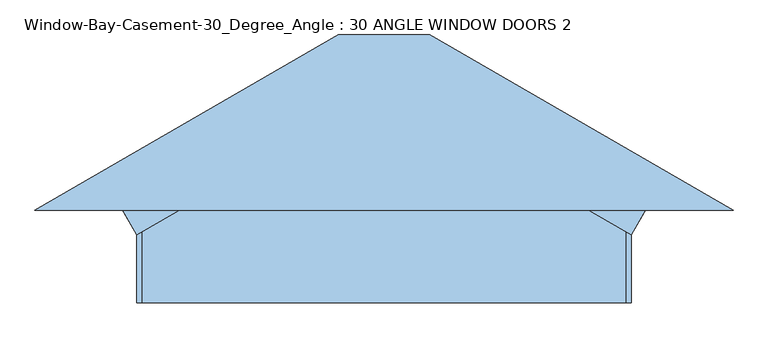
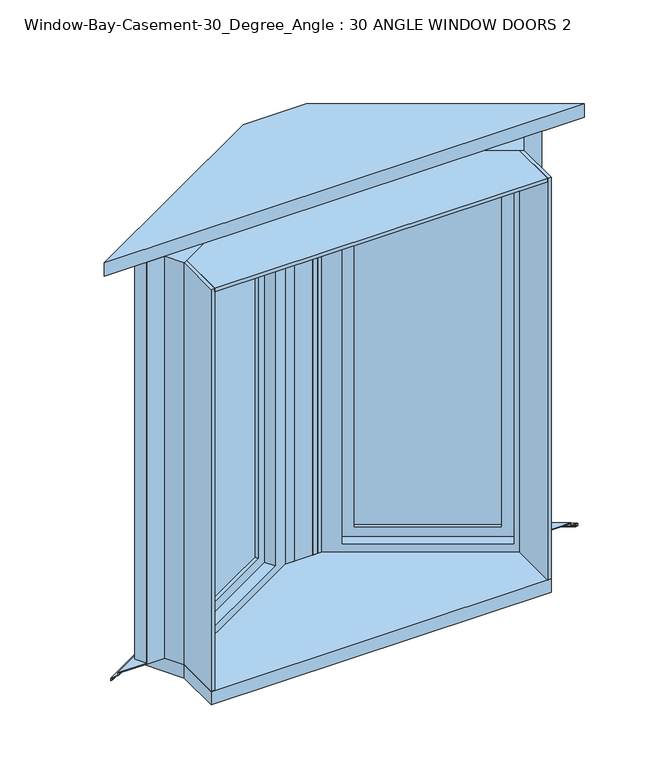
"""IFC4 building model written with IfcOpenShell, lengths in millimetres: window geometry, Window-Bay-Casement-30_Degree_Angle : 30 ANGLE WINDOW DOORS 2."""

from ifc_helpers import new_model, si_unit, frame, origin, place, context, project, spatial, polyline, outline, extrude, faceted_brep, source, transform, mapped, element, save


def window_bay_casement_30_degree_angle_30_angle_window_doors_2_b97d1700(model_context):
    return source(origin(), model_context, "Body", "SolidModel", [
        extrude(outline(polyline([(584.0331255, 149.225), (580.8581255, 143.7257387), (184.9113109, 372.3257387), (188.0863109, 377.825), (584.0331255, 149.225)])), frame((0.0, 0.0, 730.25), z_axis=(0.0, 0.0, 1.0), x_axis=(1.0, 0.0, 0.0)), (0.0, 0.0, 1.0), 1384.3),
        extrude(outline(polyline([(577.6831255, 138.2264774), (574.5081255, 132.7272161), (178.5613109, 361.3272161), (181.7363109, 366.8264774), (577.6831255, 138.2264774)])), frame((0.0, 0.0, 730.25), z_axis=(0.0, 0.0, 1.0), x_axis=(1.0, 0.0, 0.0)), (0.0, 0.0, 1.0), 1384.3),
        extrude(outline(polyline([(1441.45, 57.1500001), (1441.45, -514.35), (-57.15, -514.35), (-57.15, 57.1500001), (1441.45, 57.1500001)]), holes=[polyline([(1384.3, -457.2), (1384.3, 0.0), (0.0, 0.0), (0.0, -457.2), (1384.3, -457.2)])]), frame((568.1581255, 121.7286934, 730.25), z_axis=(0.49999999999999967, 0.8660254037844389, 0.0), x_axis=(0.0, 0.0, 1.0)), (0.0, 0.0, 1.0), 44.45),
        faceted_brep([(64.8840949, 368.3, 2184.4), (609.6, 53.8081255, 2184.4), (644.525, 114.3, 2184.4), (708.025, 114.3, 2184.4), (92.1077328, 469.9, 2184.4), (617.6514774, 93.1536934, 2171.7), (122.7179591, 378.9036934, 2171.7), (154.4679591, 433.8963066, 2171.7), (649.4014774, 148.1463066, 2171.7), (582.1036934, 69.6831255, 2152.65), (120.1657431, 336.3831255, 2152.65), (139.2157431, 369.3786934, 2152.65), (601.1536934, 102.6786934, 2152.65), (122.7179591, 378.9036934, 673.1), (154.4679591, 433.8963066, 673.1), (120.1657431, 336.3831255, 692.15), (139.2157431, 369.3786934, 692.15), (92.1077328, 469.9, 660.4), (708.025, 114.3, 660.4), (644.525, 114.3, 660.4), (609.6, 53.8081255, 660.4), (64.8840949, 368.3, 660.4), (617.6514774, 93.1536934, 673.1), (649.4014774, 148.1463066, 673.1), (582.1036934, 69.6831255, 692.15), (601.1536934, 102.6786934, 692.15)], [[[0, 1, 2, 3, 4]], [[5, 6, 7, 8]], [[9, 10, 11, 12]], [[6, 13, 14, 7]], [[10, 15, 16, 11]], [[17, 18, 19, 20, 21]], [[13, 22, 23, 14]], [[15, 24, 25, 16]], [[20, 19, 2, 1]], [[3, 18, 17, 4], [7, 14, 23, 8]], [[8, 23, 22, 5]], [[5, 22, 13, 6], [11, 16, 25, 12]], [[12, 25, 24, 9]], [[1, 0, 21, 20], [9, 24, 15, 10]], [[4, 17, 21, 0]], [[2, 19, 18, 3]]]),
        extrude(outline(polyline([(-584.0331255, 149.225), (-188.0863109, 377.825), (-184.9113109, 372.3257387), (-580.8581255, 143.7257387), (-584.0331255, 149.225)])), frame((0.0, 0.0, 730.25), z_axis=(0.0, 0.0, 1.0), x_axis=(1.0, 0.0, 0.0)), (0.0, 0.0, 1.0), 1384.3),
        extrude(outline(polyline([(-577.6831255, 138.2264774), (-181.7363109, 366.8264774), (-178.5613109, 361.3272161), (-574.5081255, 132.7272161), (-577.6831255, 138.2264774)])), frame((0.0, 0.0, 730.25), z_axis=(0.0, 0.0, 1.0), x_axis=(1.0, 0.0, 0.0)), (0.0, 0.0, 1.0), 1384.3),
        extrude(outline(polyline([(1441.45, -57.1500001), (-57.15, -57.1500001), (-57.15, 514.35), (1441.45, 514.35), (1441.45, -57.1500001)]), holes=[polyline([(1384.3, 457.2), (0.0, 457.2), (0.0, 0.0), (1384.3, 0.0), (1384.3, 457.2)])]), frame((-568.1581255, 121.7286934, 730.25), z_axis=(-0.49999999999999967, 0.8660254037844389, 0.0), x_axis=(0.0, 0.0, 1.0)), (0.0, 0.0, 1.0), 44.45),
        faceted_brep([(-64.8840949, 368.3, 2184.4), (-92.1077328, 469.9, 2184.4), (-708.025, 114.3, 2184.4), (-644.525, 114.3, 2184.4), (-609.6, 53.8081255, 2184.4), (-617.6514774, 93.1536934, 2171.7), (-649.4014774, 148.1463066, 2171.7), (-154.4679591, 433.8963066, 2171.7), (-122.7179591, 378.9036934, 2171.7), (-582.1036934, 69.6831255, 2152.65), (-601.1536934, 102.6786934, 2152.65), (-139.2157431, 369.3786934, 2152.65), (-120.1657431, 336.3831255, 2152.65), (-154.4679591, 433.8963066, 673.1), (-122.7179591, 378.9036934, 673.1), (-139.2157431, 369.3786934, 692.15), (-120.1657431, 336.3831255, 692.15), (-92.1077328, 469.9, 660.4), (-64.8840949, 368.3, 660.4), (-609.6, 53.8081255, 660.4), (-644.525, 114.3, 660.4), (-708.025, 114.3, 660.4), (-649.4014774, 148.1463066, 673.1), (-617.6514774, 93.1536934, 673.1), (-601.1536934, 102.6786934, 692.15), (-582.1036934, 69.6831255, 692.15)], [[[0, 1, 2, 3, 4]], [[5, 6, 7, 8]], [[9, 10, 11, 12]], [[8, 7, 13, 14]], [[12, 11, 15, 16]], [[17, 18, 19, 20, 21]], [[14, 13, 22, 23]], [[16, 15, 24, 25]], [[19, 4, 3, 20]], [[2, 1, 17, 21], [7, 6, 22, 13]], [[6, 5, 23, 22]], [[5, 8, 14, 23], [11, 10, 24, 15]], [[10, 9, 25, 24]], [[4, 19, 18, 0], [9, 12, 16, 25]], [[1, 0, 18, 17]], [[3, 2, 21, 20]]]),
        faceted_brep([(-105.7449774, 520.7, 660.4), (-105.7449774, 520.7, 653.0697935), (105.7449774, 520.7, 653.0697935), (105.7449774, 520.7, 660.4), (-92.1331585, 469.9, 663.1486341), (-92.1331585, 469.9, 660.4), (92.1331585, 469.9, 660.4), (92.1331585, 469.9, 663.1486341), (-106.1193025, 522.097, 654.4483503), (-106.1193025, 522.097, 663.1486341), (106.1193025, 522.097, 663.1486341), (106.1193025, 522.097, 654.4483503), (109.5222572, 534.797, 652.2089977), (-109.5222572, 534.797, 652.2089977), (109.5222572, 534.797, 643.2668038), (-109.5222572, 534.797, 643.2668038), (-108.4605353, 530.8346, 644.7270038), (-108.4605353, 530.8346, 643.2668038), (108.4605353, 530.8346, 643.2668038), (108.4605353, 530.8346, 644.7270038), (-109.0934849, 533.1968, 650.8662705), (-109.0934849, 533.1968, 644.7270038), (109.0934849, 533.1968, 644.7270038), (109.0934849, 533.1968, 650.8662705), (-809.6504256, 114.3, 660.4), (-809.6504256, 114.3, 653.0697935), (809.6504256, 114.3, 660.4), (708.0504256, 114.3, 660.4), (-708.0504256, 114.3, 660.4), (-708.0504256, 114.3, 663.1486341), (708.0504256, 114.3, 663.1486341), (812.4444256, 114.3, 663.1486341), (-812.4444256, 114.3, 663.1486341), (-812.4444256, 114.3, 654.4483503), (-837.8444256, 114.3, 652.2089977), (-837.8444256, 114.3, 643.2668038), (837.8444256, 114.3, 643.2668038), (829.9196257, 114.3, 643.2668038), (-829.9196257, 114.3, 643.2668038), (-829.9196257, 114.3, 644.7270038), (829.9196257, 114.3, 644.7270038), (834.6440256, 114.3, 644.7270038), (-834.6440256, 114.3, 644.7270038), (-834.6440256, 114.3, 650.8662705), (809.6504256, 114.3, 653.0697935), (812.4444256, 114.3, 654.4483503), (837.8444256, 114.3, 652.2089977), (834.6440256, 114.3, 650.8662705)], [[[0, 1, 2, 3]], [[4, 5, 6, 7]], [[8, 9, 10, 11]], [[8, 11, 12, 13]], [[13, 12, 14, 15]], [[16, 17, 18, 19]], [[20, 21, 22, 23]], [[2, 1, 20, 23]], [[1, 0, 24, 25]], [[0, 3, 26, 27, 6, 5, 28, 24]], [[5, 4, 29, 28]], [[4, 7, 30, 31, 10, 9, 32, 29]], [[9, 8, 33, 32]], [[8, 13, 34, 33]], [[13, 15, 35, 34]], [[15, 14, 36, 37, 18, 17, 38, 35]], [[17, 16, 39, 38]], [[16, 19, 40, 41, 22, 21, 42, 39]], [[21, 20, 43, 42]], [[20, 1, 25, 43]], [[3, 2, 44, 26]], [[7, 6, 27, 30]], [[11, 10, 31, 45]], [[12, 11, 45, 46]], [[14, 12, 46, 36]], [[19, 18, 37, 40]], [[23, 22, 41, 47]], [[2, 23, 47, 44]], [[25, 24, 28, 29, 32, 33, 34, 35, 38, 39, 42, 43]], [[27, 26, 44, 47, 41, 40, 37, 36, 46, 45, 31, 30]]]),
        extrude(outline(polyline([(-680.5541191, 130.175), (-708.0504256, 114.3), (-730.2754256, 152.7948292), (-702.7791191, 168.6698292), (-680.5541191, 130.175)])), frame((0.0, 0.0, 663.1486341), z_axis=(0.0, 0.0, 1.0), x_axis=(1.0, 0.0, 0.0)), (0.0, 0.0, 1.0), 1521.2513659),
        extrude(outline(polyline([(680.5541191, 130.175), (702.7791191, 168.6698292), (730.2754256, 152.7948292), (708.0504256, 114.3), (680.5541191, 130.175)])), frame((0.0, 0.0, 663.1486341), z_axis=(0.0, 0.0, 1.0), x_axis=(1.0, 0.0, 0.0)), (0.0, 0.0, 1.0), 1521.2513659),
        extrude(outline(polyline([(112.5254613, 546.1), (860.425, 114.3), (-860.425, 114.3), (-112.5254613, 546.1), (112.5254613, 546.1)])), frame((0.0, 0.0, 2184.4), z_axis=(0.0, 0.0, 1.0), x_axis=(1.0, 0.0, 0.0)), (0.0, 0.0, 1.0), 50.8),
        extrude(outline(polyline([(-32.800346, 469.9), (-32.800346, 368.3), (-64.8840949, 368.3), (-92.1077328, 469.9), (-32.800346, 469.9)])), frame((0.0, 0.0, 660.4), z_axis=(0.0, 0.0, 1.0), x_axis=(1.0, 0.0, 0.0)), (0.0, 0.0, 1.0), 1524.0),
        extrude(outline(polyline([(92.1077328, 469.9), (64.8840949, 368.3), (32.800346, 368.3), (32.800346, 469.9), (92.1077328, 469.9)])), frame((0.0, 0.0, 660.4), z_axis=(0.0, 0.0, 1.0), x_axis=(1.0, 0.0, 0.0)), (0.0, 0.0, 1.0), 1524.0),
        extrude(outline(polyline([(50.8, 469.9), (50.8, 368.3), (-50.8, 368.3), (-50.8, 469.9), (50.8, 469.9)])), frame((0.0, 0.0, 660.4), z_axis=(0.0, 0.0, 1.0), x_axis=(1.0, 0.0, 0.0)), (0.0, 0.0, 1.0), 1524.0),
        faceted_brep([(-63.5, 406.4, 647.7), (-63.5, 469.9, 647.7), (-20.100346, 469.9, 647.7), (-20.100346, 406.4, 647.7), (-82.55, 368.3, 628.65), (-82.55, 406.4, 628.65), (-1.050346, 406.4, 628.65), (-1.050346, 368.3, 628.65), (-50.8, 469.9, 660.4), (-50.8, 368.3, 660.4), (-32.800346, 368.3, 660.4), (-32.800346, 469.9, 660.4), (-20.100346, 469.9, 2197.1), (-20.100346, 406.4, 2197.1), (-1.050346, 406.4, 2216.15), (-1.050346, 368.3, 2216.15), (-32.800346, 368.3, 2184.4), (-32.800346, 469.9, 2184.4), (-63.5, 469.9, 2197.1), (-63.5, 406.4, 2197.1), (-82.55, 406.4, 2216.15), (-82.55, 368.3, 2216.15), (-50.8, 368.3, 2184.4), (-50.8, 469.9, 2184.4)], [[[0, 1, 2, 3]], [[4, 5, 6, 7]], [[8, 9, 10, 11]], [[3, 2, 12, 13]], [[7, 6, 14, 15]], [[11, 10, 16, 17]], [[13, 12, 18, 19]], [[15, 14, 20, 21]], [[17, 16, 22, 23]], [[1, 18, 12, 2], [11, 17, 23, 8]], [[19, 18, 1, 0]], [[5, 20, 14, 6], [3, 13, 19, 0]], [[21, 20, 5, 4]], [[7, 15, 21, 4], [9, 22, 16, 10]], [[23, 22, 9, 8]]]),
        extrude(outline(polyline([(-120.65, 438.15), (37.049654, 438.15), (37.049654, 431.8), (-120.65, 431.8), (-120.65, 438.15)])), frame((0.0, 0.0, 730.25), z_axis=(0.0, 0.0, 1.0), x_axis=(1.0, 0.0, 0.0)), (0.0, 0.0, 1.0), 1384.3),
        extrude(outline(polyline([(-120.65, 425.45), (37.049654, 425.45), (37.049654, 419.1), (-120.65, 419.1), (-120.65, 425.45)])), frame((0.0, 0.0, 730.25), z_axis=(0.0, 0.0, 1.0), x_axis=(1.0, 0.0, 0.0)), (0.0, 0.0, 1.0), 1384.3),
        extrude(outline(polyline([(-37.049654, 438.15), (120.65, 438.15), (120.65, 431.8), (-37.049654, 431.8), (-37.049654, 438.15)])), frame((0.0, 0.0, 730.25), z_axis=(0.0, 0.0, 1.0), x_axis=(1.0, 0.0, 0.0)), (0.0, 0.0, 1.0), 1384.3),
        extrude(outline(polyline([(-37.049654, 425.45), (120.65, 425.45), (120.65, 419.1), (-37.049654, 419.1), (-37.049654, 425.45)])), frame((0.0, 0.0, 730.25), z_axis=(0.0, 0.0, 1.0), x_axis=(1.0, 0.0, 0.0)), (0.0, 0.0, 1.0), 1384.3),
        faceted_brep([(20.100346, 406.4, 647.7), (20.100346, 469.9, 647.7), (63.5, 469.9, 647.7), (63.5, 406.4, 647.7), (1.050346, 368.3, 628.65), (1.050346, 406.4, 628.65), (82.55, 406.4, 628.65), (82.55, 368.3, 628.65), (32.800346, 469.9, 660.4), (32.800346, 368.3, 660.4), (50.8, 368.3, 660.4), (50.8, 469.9, 660.4), (63.5, 469.9, 2197.1), (63.5, 406.4, 2197.1), (82.55, 406.4, 2216.15), (82.55, 368.3, 2216.15), (50.8, 368.3, 2184.4), (50.8, 469.9, 2184.4), (20.100346, 469.9, 2197.1), (20.100346, 406.4, 2197.1), (1.050346, 406.4, 2216.15), (1.050346, 368.3, 2216.15), (32.800346, 368.3, 2184.4), (32.800346, 469.9, 2184.4)], [[[0, 1, 2, 3]], [[4, 5, 6, 7]], [[8, 9, 10, 11]], [[3, 2, 12, 13]], [[7, 6, 14, 15]], [[11, 10, 16, 17]], [[13, 12, 18, 19]], [[15, 14, 20, 21]], [[17, 16, 22, 23]], [[1, 18, 12, 2], [11, 17, 23, 8]], [[19, 18, 1, 0]], [[5, 20, 14, 6], [3, 13, 19, 0]], [[21, 20, 5, 4]], [[7, 15, 21, 4], [9, 22, 16, 10]], [[23, 22, 9, 8]]]),
        extrude(outline(polyline([(609.6, -114.3), (-609.6, -114.3), (-609.6, 53.8081255), (-685.8, 185.7903971), (-105.7195518, 520.7), (105.7195518, 520.7), (685.8, 185.7903971), (609.6, 53.8081256), (609.6, -114.3)])), frame((0.0, 0.0, 609.6), z_axis=(0.0, 0.0, 1.0), x_axis=(1.0, 0.0, 0.0)), (0.0, 0.0, 1.0), 50.8),
        extrude(outline(polyline([(2228.85, -37.049654), (615.95, -37.049654), (615.95, 120.65), (2228.85, 120.65), (2228.85, -37.049654)]), holes=[polyline([(2171.7, 63.5), (673.1, 63.5), (673.1, 20.100346), (2171.7, 20.100346), (2171.7, 63.5)])]), frame((0.0, 406.4, 0.0), z_axis=(0.0, 1.0, 0.0), x_axis=(0.0, 0.0, 1.0)), (0.0, 0.0, 1.0), 44.45),
        extrude(outline(polyline([(2228.85, -120.65), (590.55, -120.65), (590.55, 37.049654), (2228.85, 37.049654), (2228.85, -120.65)]), holes=[polyline([(2171.7, -20.100346), (647.7, -20.100346), (647.7, -63.5), (2171.7, -63.5), (2171.7, -20.100346)])]), frame((0.0, 406.4, 0.0), z_axis=(0.0, 1.0, 0.0), x_axis=(0.0, 0.0, 1.0)), (0.0, 0.0, 1.0), 44.45),
        extrude(outline(polyline([(-609.6, -114.3), (-609.6, 53.8081255), (-596.9, 61.140474), (-596.9, -114.3), (-609.6, -114.3)])), frame((0.0, 0.0, 660.4), z_axis=(0.0, 0.0, 1.0), x_axis=(1.0, 0.0, 0.0)), (0.0, 0.0, 1.0), 1524.0),
        extrude(outline(polyline([(609.6, -114.3), (596.9, -114.3), (596.9, 61.140474), (609.6, 53.8081256), (609.6, -114.3)])), frame((0.0, 0.0, 660.4), z_axis=(0.0, 0.0, 1.0), x_axis=(1.0, 0.0, 0.0)), (0.0, 0.0, 1.0), 1524.0),
        extrude(outline(polyline([(-64.8840949, 368.3), (64.8840949, 368.3), (596.9, 61.140474), (596.9, -114.3), (-596.9, -114.3), (-596.9, 61.140474), (-64.8840949, 368.3)])), frame((0.0, 0.0, 2171.7), z_axis=(0.0, 0.0, 1.0), x_axis=(1.0, 0.0, 0.0)), (0.0, 0.0, 1.0), 12.7),
    ])


if __name__ == "__main__":
    model = new_model("IFC4")
    model_context = context("Model", 3, world=origin())
    ifc_project = project(units=[si_unit("LENGTHUNIT", "METRE", prefix="MILLI")], contexts=[model_context])
    site = spatial("IfcSite", under=ifc_project)
    building = spatial("IfcBuilding", under=site)
    placement = place(None, origin())
    window_bay_casement_30_degree_angle_30_angle_window_doors_2_shape = window_bay_casement_30_degree_angle_30_angle_window_doors_2_b97d1700(model_context)
    element("IfcWindow", 1, ObjectType="Window-Bay-Casement-30_Degree_Angle : 30 ANGLE WINDOW DOORS 2", at=placement, inside=building, context=model_context, shape_type="MappedRepresentation", body=[
        mapped(window_bay_casement_30_degree_angle_30_angle_window_doors_2_shape, transform((0.0, 0.0, 0.0), x_axis=(1.0, 0.0, 0.0), y_axis=(0.0, 1.0, 0.0), z_axis=(0.0, 0.0, 1.0))),
    ])
    save(model, "model.ifc")

# Revit data of these elements
# Type "Window-Bay-Casement-30_Degree_Angle : 30 ANGLE WINDOW DOORS 2"
#   Type Mark = "20"
#   Fire Rating = "0.5h"
#   Assembly Code = "B2020100"
#   Analytic Construction = "Double glazing - domestic"
#   Width of Middle Sash = 0' - 2.5827"
#   Width = 4' - 0"
#   Visual Light Transmittance = 0.81
#   Thermal Resistance (R) = 1.8146 (h·ft²·°F)/BTU
#   Solar Heat Gain Coefficient = 0.76
#   Rough Width = 4' - 0 1/2"
#   Rough Height = 5' - 0 1/2"
#   Length 2 = 0' - 7.25458"
#   Length 1 = 1' - 8.70865"
#   Wall Thickness [instance default] = 0' - 6"
#   Trim Width = 4' - 4 43/64"
#   Trim Height = 5' - 0"
#   Height 1 = 5' - 2"
#   Height = 5' - 0"
#   Heat Transfer Coefficient (U) = 0.5511 BTU/(h·ft²·°F)
#   Depth = 1' - 2"
#   Default Sill Height = 2' - 0"
#   Angle = 30.00°
#   Muntin Visibility = yes
#   Interior Trim Visibility [instance default] = yes
#   Exterior Trim Visibility [instance default] = yes
#   Muntin Pattern = Muntin Pattern_2x2 : Muntin Pattern_2x2
#   Interior Trim Material = Wood - Stained
#   Exterior Trim Material = Clad - White
#   Exterior Trim = element 398720
#   Interior Trim = Trim-Window-Interior-Flat : Picture Frame
#   Interior Frame Material = Wood - Stained
#   Glass Panel Material = Glass
#   Exterior Frame Material = Clad - White
#   Wall Closure = (empty or 0)
# Element 1 (IfcWindow, "Window-Bay-Casement-30_Degree_Angle : 30 ANGLE WINDOW DOORS 2")
#   Wall Thickness = 0' - 9"
#   Materials on its faces: "Clad - White", "Wood - Stained", "Glass"
# Materials
#   "Wood - Stained": class "Wood", colour RGB 224 178 126, transparency 0, Cost = 0
#   "Clad - White": class "Wood", colour RGB 30 30 30, transparency 0, Cost = 0
#   "Glass": class "Glass", colour RGB 0 128 192, transparency 0.75, Description = "Soda Lime Glass", Cost = 0
